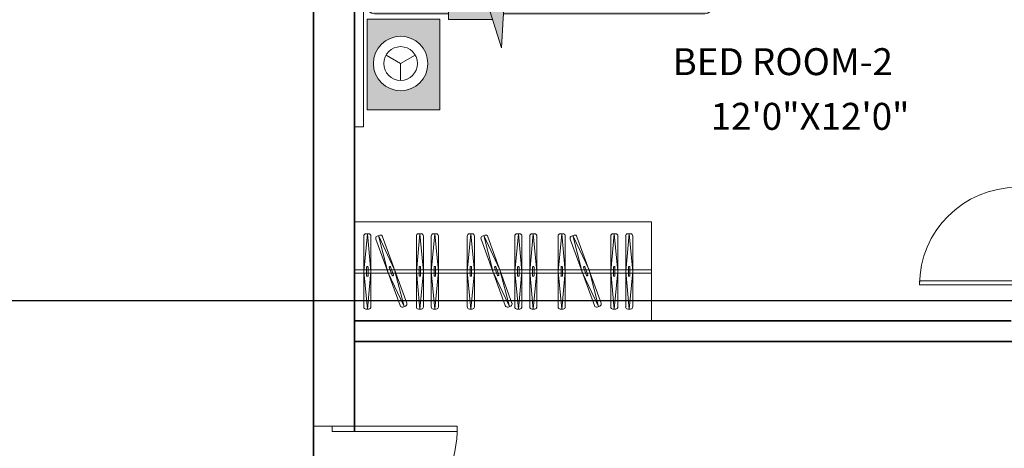
# Model space of a CAD drawing. Units: millimetres. Extents: x 27017497 to 27018854, y 7058029 to 7059154.
# Tile 79 of 91: x 27018246 to 27018462, y 7058409 to 7058503. Entities that reach past the tile are written whole.
import ezdxf

# ---------------------------------------------------------------- set-up
doc = ezdxf.new("R2010")
doc.units = ezdxf.units.MM
for name, color, linetype, lineweight in [('A-ANNO-DIMS', 2, 'Continuous', 18), ('A-AREA-IDEN', 7, 'Continuous', 18), ('A-DOOR', 4, 'Continuous', 20), ('A-FLOR-CASE', 8, 'Continuous', 20), ('A-FURN', 8, 'Continuous', 18), ('A-WALL', 7, 'Continuous', 35)]:
    doc.layers.add(name, color=color, linetype=linetype, lineweight=lineweight)
doc.layers.add('A-FURN-PATT', color=177, linetype='Continuous', lineweight=13, true_color=0x293189)
doc.styles.get("Standard").update_dxf_attribs({"font": 'arial.ttf'})
doc.dimstyles.get("Standard").update_dxf_attribs({"dimtxt": 0.18, "dimasz": 0.18, "dimexe": 0.18, "dimexo": 0.0625, "dimgap": 0.09, "dimtad": 0, "dimtih": 1, "dimtoh": 1, "dimdec": 4, "dimzin": 0, "dimdsep": 46, "dimtxsty": 'Standard', "dimcen": 0.09, "dimadec": 0, "dimazin": 0, "dimtfac": 1, "dimtdec": 4, "dimtofl": 0, "dimtmove": 0, "dimatfit": 3, "dimfxl": 1, "dimtolj": 1, "dimtzin": 0, "dimarcsym": 0})

# ---------------------------------------------------------------- blocks, each defined once
blk = doc.blocks.new('CAMMAT')
for p, q in [((1.2731, 0), (-1.2731, 0)), ((1.2731, 0), (1.2731, -0.05)), ((-1.2731, 0), (-1.2731, -0.05)), ((1.2731, -0.05), (-1.2731, -0.05)), ((-1.18, -0.07), (-1.18, -0.47)), ((-1.18, -0.07), (-0.68, -0.07)), ((-0.68, -0.07), (-0.68, -0.47)), ((0.61, -0.07), (-0.61, -0.07)), ((0.68, -0.07), (0.68, -0.47)), ((0.68, -0.07), (1.18, -0.07)), ((1.18, -0.07), (1.18, -0.47)), ((-0.65, -0.11), (-0.65, -0.5169)), ((-0.0465, -0.1395), (-0.5852, -0.1395)), ((0.5962, -0.1395), (0.0574, -0.1395)), ((0.65, -0.11), (0.65, -0.5169)), ((-0.931, -0.2541), (-0.9775, -0.1737)), ((-0.6152, -0.1695), (-0.6152, -0.4095)), ((-0.0165, -0.1695), (-0.0165, -0.4095)), ((0.0274, -0.1695), (0.0274, -0.4095)), ((0.6262, -0.1695), (0.6262, -0.4095)), ((0.9242, -0.2541), (0.8777, -0.1737)), ((-0.931, -0.2541), (-0.9775, -0.3346)), ((-0.931, -0.2541), (-0.8381, -0.2541)), ((0.9242, -0.2541), (0.8777, -0.3346)), ((0.9242, -0.2541), (1.0171, -0.2541)), ((-1.18, -0.47), (-0.68, -0.47)), ((-0.0465, -0.4395), (-0.5852, -0.4395)), ((0.5962, -0.4395), (0.0574, -0.4395)), ((0.68, -0.47), (1.18, -0.47)), ((-0.6904, -0.5169), (-0.6904, -0.8)), ((-0.6904, -0.5169), (0.6826, -0.5169)), ((0.6826, -0.5169), (0.6826, -0.7603)), ((0.0535, -0.5623), (-0.7312, -0.8093)), ((0.0535, -0.5623), (0.8382, -0.8093)), ((-0.65, -0.8139), (-0.65, -1.93)), ((0.65, -0.8204), (0.65, -1.93)), ((0.61, -1.97), (-0.61, -1.97))]:
    blk.add_line(p, q)
for points in [[(-0.1761, -1.0476), (-0.161, -0.9772), (-0.1474, -0.921), (-0.1326, -0.8732), (-0.1139, -0.8282), (-0.0886, -0.7803), (-0.0541, -0.7238), (-0.0076, -0.653), (0.0535, -0.5623)], [(0.2832, -1.0476), (0.2681, -0.9772), (0.2545, -0.921), (0.2396, -0.8732), (0.2209, -0.8282), (0.1957, -0.7803), (0.1611, -0.7238), (0.1147, -0.653), (0.0535, -0.5623)], [(-0.7312, -0.8093), (-0.5683, -0.8185), (-0.4451, -0.828), (-0.3552, -0.8406), (-0.2919, -0.8591), (-0.2489, -0.8862), (-0.2196, -0.9248), (-0.1975, -0.9777), (-0.1761, -1.0476)], [(0.8382, -0.8093), (0.6753, -0.8185), (0.5522, -0.828), (0.4622, -0.8406), (0.399, -0.8591), (0.356, -0.8862), (0.3267, -0.9248), (0.3046, -0.9777), (0.2832, -1.0476)]]:
    blk.add_lwpolyline(points)
for centre, radius in [((-0.931, -0.2541), 0.15), ((0.9242, -0.2541), 0.15), ((-0.931, -0.2541), 0.0929), ((0.9242, -0.2541), 0.0929)]:
    blk.add_circle(centre, radius)
for centre, radius, start, end in [((-0.61, -0.11), 0.04, 90, 180), ((0.61, -0.11), 0.04, 0, 90), ((-0.5852, -0.1695), 0.03, 90, 180), ((-0.0465, -0.1695), 0.03, 360, 90), ((0.0574, -0.1695), 0.03, 90, 180), ((0.5962, -0.1695), 0.03, 360, 90), ((-0.5852, -0.4095), 0.03, 180, 270), ((-0.0465, -0.4095), 0.03, 270, 360), ((0.0574, -0.4095), 0.03, 180, 270), ((0.5962, -0.4095), 0.03, 270, 360), ((-0.61, -1.93), 0.04, 180, 270), ((0.61, -1.93), 0.04, 270, 360)]:
    blk.add_arc(centre, radius, start, end)
blk = doc.blocks.new('*U2')
for p, q in [((0, 0), (0, -6)), ((40, 0), (40, -6))]:
    blk.add_line(p, q)
blk.add_lwpolyline([(0, 0), (0, 40), (1.75, 40), (1.75, 0)], close=True)
blk.add_arc((0, 0), 40, 0, 90)
blk = doc.blocks.new('WARDROBE-HANGING')
for p, q in [((0, 21.74), (65.21, 21.74)), ((0, 0), (0, 21.74)), ((65.21, 0), (65.21, 21.74)), ((4.86, 19.15), (4.08, 10.88)), ((4.08, 18.62), (4.08, 3.13)), ((5.18, 19.15), (4.55, 19.15)), ((4.86, 19.15), (5.64, 10.88)), ((5.64, 18.62), (5.64, 3.13)), ((8.14, 19.15), (7.35, 10.88)), ((7.35, 18.62), (7.35, 3.13)), ((8.45, 19.15), (7.82, 19.15)), ((8.14, 19.15), (8.92, 10.88)), ((8.92, 18.62), (8.92, 3.13)), ((16.33, 18.5), (11.03, 3.94)), ((17.8, 17.96), (12.5, 3.4)), ((17.25, 18.73), (13.68, 11.22)), ((17.25, 18.73), (15.15, 10.68)), ((17.54, 18.62), (16.95, 18.83)), ((19.66, 19.15), (18.88, 10.88)), ((18.88, 18.62), (18.88, 3.13)), ((19.98, 19.15), (19.35, 19.15)), ((19.66, 19.15), (20.45, 10.88)), ((20.45, 18.62), (20.45, 3.13)), ((25.9, 19.15), (25.12, 10.88)), ((25.12, 18.62), (25.12, 3.13)), ((26.21, 19.15), (25.59, 19.15)), ((25.9, 19.15), (26.68, 10.88)), ((26.68, 18.62), (26.68, 3.13)), ((29.17, 19.15), (28.39, 10.88)), ((28.39, 18.62), (28.39, 3.13)), ((29.49, 19.15), (28.86, 19.15)), ((29.17, 19.15), (29.96, 10.88)), ((29.96, 18.62), (29.96, 3.13)), ((35.87, 18.5), (30.57, 3.94)), ((37.34, 17.96), (32.04, 3.4)), ((36.78, 18.73), (33.22, 11.22)), ((36.78, 18.73), (34.69, 10.68)), ((37.08, 18.62), (36.49, 18.83)), ((39.59, 19.15), (38.81, 10.88)), ((38.81, 18.62), (38.81, 3.13)), ((39.9, 19.15), (39.28, 19.15)), ((39.59, 19.15), (40.37, 10.88)), ((40.37, 18.62), (40.37, 3.13)), ((47.49, 19.15), (46.71, 10.88)), ((46.71, 18.62), (46.71, 3.13)), ((47.81, 19.15), (47.18, 19.15)), ((47.49, 19.15), (48.28, 10.88)), ((48.28, 18.62), (48.28, 3.13)), ((50.77, 19.15), (49.98, 10.88)), ((49.98, 18.62), (49.98, 3.13)), ((51.08, 19.15), (50.45, 19.15)), ((50.77, 19.15), (51.55, 10.88)), ((51.55, 18.62), (51.55, 3.13)), ((58.96, 18.5), (53.66, 3.94)), ((60.43, 17.96), (55.13, 3.4)), ((59.88, 18.73), (56.31, 11.22)), ((59.88, 18.73), (57.78, 10.68)), ((60.17, 18.62), (59.58, 18.83)), ((62.29, 19.15), (61.51, 10.88)), ((61.51, 18.62), (61.51, 3.13)), ((62.61, 19.15), (61.98, 19.15)), ((62.29, 19.15), (63.08, 10.88)), ((63.08, 18.62), (63.08, 3.13)), ((0, 11.23), (65.21, 11.23)), ((4.86, 2.6), (4.08, 10.88)), ((4.71, 11.83), (4.71, 9.93)), ((4.92, 11.93), (4.8, 11.93)), ((4.86, 2.6), (5.64, 10.88)), ((5.02, 11.83), (5.02, 9.93)), ((8.14, 2.6), (7.35, 10.88)), ((7.98, 11.83), (7.98, 9.93)), ((8.2, 11.93), (8.07, 11.93)), ((8.14, 2.6), (8.92, 10.88)), ((8.29, 11.83), (8.29, 9.93)), ((11.59, 3.17), (13.68, 11.22)), ((14.59, 11.9), (13.94, 10.11)), ((14.89, 11.79), (14.24, 10)), ((14.84, 11.92), (14.72, 11.96)), ((19.66, 2.6), (18.88, 10.88)), ((19.51, 11.83), (19.51, 9.93)), ((19.73, 11.93), (19.6, 11.93)), ((19.66, 2.6), (20.45, 10.88)), ((19.82, 11.83), (19.82, 9.93)), ((25.9, 2.6), (25.12, 10.88)), ((25.74, 11.83), (25.74, 9.93)), ((25.96, 11.93), (25.84, 11.93)), ((25.9, 2.6), (26.68, 10.88)), ((26.06, 11.83), (26.06, 9.93)), ((29.17, 2.6), (28.39, 10.88)), ((29.02, 11.83), (29.02, 9.93)), ((29.24, 11.93), (29.11, 11.93)), ((29.17, 2.6), (29.96, 10.88)), ((29.33, 11.83), (29.33, 9.93)), ((31.12, 3.17), (33.22, 11.22)), ((34.13, 11.9), (33.48, 10.11)), ((34.42, 11.79), (33.77, 10)), ((34.37, 11.92), (34.25, 11.96)), ((39.59, 2.6), (38.81, 10.88)), ((39.43, 11.83), (39.43, 9.93)), ((39.65, 11.93), (39.53, 11.93)), ((39.59, 2.6), (40.37, 10.88)), ((39.75, 11.83), (39.75, 9.93)), ((47.49, 2.6), (46.71, 10.88)), ((47.34, 11.83), (47.34, 9.93)), ((47.56, 11.93), (47.43, 11.93)), ((47.49, 2.6), (48.28, 10.88)), ((47.65, 11.83), (47.65, 9.93)), ((50.77, 2.6), (49.98, 10.88)), ((50.61, 11.83), (50.61, 9.93)), ((50.83, 11.93), (50.7, 11.93)), ((50.77, 2.6), (51.55, 10.88)), ((50.92, 11.83), (50.92, 9.93)), ((54.22, 3.17), (56.31, 11.22)), ((57.22, 11.9), (56.57, 10.11)), ((57.52, 11.79), (56.87, 10)), ((57.47, 11.92), (57.35, 11.96)), ((62.29, 2.6), (61.51, 10.88)), ((62.14, 11.83), (62.14, 9.93)), ((62.36, 11.93), (62.23, 11.93)), ((62.29, 2.6), (63.08, 10.88)), ((62.45, 11.83), (62.45, 9.93)), ((0, 10.51), (65.21, 10.51)), ((4.92, 9.82), (4.8, 9.82)), ((8.2, 9.82), (8.07, 9.82)), ((11.59, 3.17), (15.15, 10.68)), ((14.11, 9.94), (14, 9.98)), ((19.73, 9.82), (19.6, 9.82)), ((25.96, 9.82), (25.84, 9.82)), ((29.24, 9.82), (29.11, 9.82)), ((31.12, 3.17), (34.69, 10.68)), ((33.65, 9.94), (33.53, 9.98)), ((39.65, 9.82), (39.53, 9.82)), ((47.56, 9.82), (47.43, 9.82)), ((50.83, 9.82), (50.7, 9.82)), ((54.22, 3.17), (57.78, 10.68)), ((56.74, 9.94), (56.63, 9.98)), ((62.36, 9.82), (62.23, 9.82)), ((5.18, 2.6), (4.55, 2.6)), ((8.45, 2.6), (7.82, 2.6)), ((11.88, 3.07), (11.29, 3.28)), ((19.98, 2.6), (19.35, 2.6)), ((26.21, 2.6), (25.59, 2.6)), ((29.49, 2.6), (28.86, 2.6)), ((31.42, 3.07), (30.83, 3.28)), ((39.9, 2.6), (39.28, 2.6)), ((47.81, 2.6), (47.18, 2.6)), ((51.08, 2.6), (50.45, 2.6)), ((54.51, 3.07), (53.92, 3.28)), ((62.61, 2.6), (61.98, 2.6)), ((0, 0), (65.21, 0))]:
    blk.add_line(p, q)
for centre, major_axis, start_param, end_param in [((4.55, 18.62), (0, 0.528), 0, 1.570796), ((5.18, 18.62), (0, 0.528), 4.712389, 6.283185), ((7.82, 18.62), (0, 0.528), 0, 1.570796), ((8.45, 18.62), (0, 0.528), 4.712389, 6.283185), ((16.77, 18.34), (0.181, 0.496), 0, 1.570796), ((17.36, 18.12), (0.181, 0.496), -1.570796, 0), ((19.35, 18.62), (0, 0.528), 0, 1.570796), ((19.98, 18.62), (0, 0.528), 4.712389, 6.283185), ((25.59, 18.62), (0, 0.528), 0, 1.570796), ((26.21, 18.62), (0, 0.528), 4.712389, 6.283185), ((28.86, 18.62), (0, 0.528), 0, 1.570796), ((29.49, 18.62), (0, 0.528), 4.712389, 6.283185), ((36.31, 18.34), (0.181, 0.496), 0, 1.570796), ((36.9, 18.12), (0.181, 0.496), -1.570796, 0), ((39.28, 18.62), (0, 0.528), 0, 1.570796), ((39.9, 18.62), (0, 0.528), 4.712389, 6.283185), ((47.18, 18.62), (0, 0.528), 0, 1.570796), ((47.81, 18.62), (0, 0.528), 4.712389, 6.283185), ((50.45, 18.62), (0, 0.528), 0, 1.570796), ((51.08, 18.62), (0, 0.528), 4.712389, 6.283185), ((59.4, 18.34), (0.181, 0.496), 0, 1.570796), ((59.99, 18.12), (0.181, 0.496), -1.570796, 0), ((61.98, 18.62), (0, 0.528), 0, 1.570796), ((62.61, 18.62), (0, 0.528), 4.712389, 6.283185), ((4.8, 11.83), (0, 0.106), 0, 1.570796), ((4.92, 11.83), (0, 0.106), -1.570796, 0), ((8.07, 11.83), (0, 0.106), 0, 1.570796), ((8.2, 11.83), (0, 0.106), -1.570796, 0), ((14.68, 11.86), (0.0361, 0.0993), 0, 1.570796), ((14.8, 11.82), (0.0361, 0.0993), 4.712389, 6.283185), ((19.6, 11.83), (0, 0.106), 0, 1.570796), ((19.73, 11.83), (0, 0.106), -1.570796, 0), ((25.84, 11.83), (0, 0.106), 0, 1.570796), ((25.96, 11.83), (0, 0.106), -1.570796, 0), ((29.11, 11.83), (0, 0.106), 0, 1.570796), ((29.24, 11.83), (0, 0.106), -1.570796, 0), ((34.22, 11.86), (0.0361, 0.0993), 0, 1.570796), ((34.34, 11.82), (0.0361, 0.0993), 4.712389, 6.283185), ((39.53, 11.83), (0, 0.106), 0, 1.570796), ((39.65, 11.83), (0, 0.106), -1.570796, 0), ((47.43, 11.83), (0, 0.106), 0, 1.570796), ((47.56, 11.83), (0, 0.106), -1.570796, 0), ((50.7, 11.83), (0, 0.106), 0, 1.570796), ((50.83, 11.83), (0, 0.106), -1.570796, 0), ((57.31, 11.86), (0.0361, 0.0993), 0, 1.570796), ((57.43, 11.82), (0.0361, 0.0993), 4.712389, 6.283185), ((62.23, 11.83), (0, 0.106), 0, 1.570796), ((62.36, 11.83), (0, 0.106), -1.570796, 0), ((4.8, 9.93), (0, 0.106), 1.570796, 3.141593), ((4.92, 9.93), (0, 0.106), 3.141593, 4.712389), ((8.07, 9.93), (0, 0.106), 1.570796, 3.141593), ((8.2, 9.93), (0, 0.106), 3.141593, 4.712389), ((14.03, 10.08), (0.0361, 0.0993), 1.570796, 3.141593), ((14.15, 10.03), (0.0361, 0.0993), 3.141593, 4.712389), ((19.6, 9.93), (0, 0.106), 1.570796, 3.141593), ((19.73, 9.93), (0, 0.106), 3.141593, 4.712389), ((25.84, 9.93), (0, 0.106), 1.570796, 3.141593), ((25.96, 9.93), (0, 0.106), 3.141593, 4.712389), ((29.11, 9.93), (0, 0.106), 1.570796, 3.141593), ((29.24, 9.93), (0, 0.106), 3.141593, 4.712389), ((33.57, 10.08), (0.0361, 0.0993), 1.570796, 3.141593), ((33.69, 10.03), (0.0361, 0.0993), 3.141593, 4.712389), ((39.53, 9.93), (0, 0.106), 1.570796, 3.141593), ((39.65, 9.93), (0, 0.106), 3.141593, 4.712389), ((47.43, 9.93), (0, 0.106), 1.570796, 3.141593), ((47.56, 9.93), (0, 0.106), 3.141593, 4.712389), ((50.7, 9.93), (0, 0.106), 1.570796, 3.141593), ((50.83, 9.93), (0, 0.106), 3.141593, 4.712389), ((56.66, 10.08), (0.0361, 0.0993), 1.570796, 3.141593), ((56.78, 10.03), (0.0361, 0.0993), 3.141593, 4.712389), ((62.23, 9.93), (0, 0.106), 1.570796, 3.141593), ((62.36, 9.93), (0, 0.106), 3.141593, 4.712389), ((4.55, 3.13), (0, 0.528), 1.570796, 3.141593), ((5.18, 3.13), (0, 0.528), 3.141593, 4.712389), ((7.82, 3.13), (0, 0.528), 1.570796, 3.141593), ((8.45, 3.13), (0, 0.528), 3.141593, 4.712389), ((11.47, 3.78), (0.181, 0.496), 1.570796, 3.141593), ((12.06, 3.56), (0.181, 0.496), 3.141593, 4.712389), ((19.35, 3.13), (0, 0.528), 1.570796, 3.141593), ((19.98, 3.13), (0, 0.528), 3.141593, 4.712389), ((25.59, 3.13), (0, 0.528), 1.570796, 3.141593), ((26.21, 3.13), (0, 0.528), 3.141593, 4.712389), ((28.86, 3.13), (0, 0.528), 1.570796, 3.141593), ((29.49, 3.13), (0, 0.528), 3.141593, 4.712389), ((31.01, 3.78), (0.181, 0.496), 1.570796, 3.141593), ((31.6, 3.56), (0.181, 0.496), 3.141593, 4.712389), ((39.28, 3.13), (0, 0.528), 1.570796, 3.141593), ((39.9, 3.13), (0, 0.528), 3.141593, 4.712389), ((47.18, 3.13), (0, 0.528), 1.570796, 3.141593), ((47.81, 3.13), (0, 0.528), 3.141593, 4.712389), ((50.45, 3.13), (0, 0.528), 1.570796, 3.141593), ((51.08, 3.13), (0, 0.528), 3.141593, 4.712389), ((54.1, 3.78), (0.181, 0.496), 1.570796, 3.141593), ((54.69, 3.56), (0.181, 0.496), 3.141593, 4.712389), ((61.98, 3.13), (0, 0.528), 1.570796, 3.141593), ((62.61, 3.13), (0, 0.528), 3.141593, 4.712389)]:
    blk.add_ellipse(centre, major_axis=major_axis, ratio=0.888892, start_param=start_param, end_param=end_param)
blk = doc.blocks.new('*D48')
at = {"layer": 'A-ANNO-DIMS', "color": 0, "lineweight": -2, "transparency": 16777216}
for p, q in [((27018463.5, 7058622.91), (27017497.54, 7058622.91)), ((27017497.72, 7058622.73), (27017497.72, 7058357.75)), ((27017497.72, 7058092.41), (27017497.72, 7058357.39)), ((27018555.13, 7058092.23), (27017497.54, 7058092.23))]:
    blk.add_line(p, q, dxfattribs=at)
at = {"layer": 'A-ANNO-DIMS', "color": 0, "transparency": 16777216}
for points in [[(27017497.69, 7058622.73), (27017497.75, 7058622.73), (27017497.72, 7058622.91)], [(27017497.69, 7058092.41), (27017497.75, 7058092.41), (27017497.72, 7058092.23)]]:
    blk.add_solid(points, dxfattribs=at)
at = {"layer": 'Defpoints', "color": 0, "transparency": 16777216}
for p in [(27018463.56, 7058622.91), (27017497.72, 7058092.23), (27018555.19, 7058092.23)]:
    blk.add_point(p, dxfattribs=at)
at = {"layer": 'A-ANNO-DIMS', "color": 0, "transparency": 16777216, "insert": (27017497.72, 7058357.57), "char_height": 0.18, "attachment_point": 5}
blk.add_mtext('\\A1;530.7', dxfattribs=at)
blk = doc.blocks.new('*D50')
at = {"layer": 'A-ANNO-DIMS', "color": 0, "lineweight": -2, "transparency": 16777216}
for p, q in [((27018223.67, 7058580.91), (27018854.24, 7058580.91)), ((27018854.06, 7058580.73), (27018854.06, 7058511.34)), ((27018854.06, 7058441.59), (27018854.06, 7058510.98)), ((27018223.67, 7058441.41), (27018854.24, 7058441.41))]:
    blk.add_line(p, q, dxfattribs=at)
at = {"layer": 'A-ANNO-DIMS', "color": 0, "transparency": 16777216}
for points in [[(27018854.03, 7058580.73), (27018854.09, 7058580.73), (27018854.06, 7058580.91)], [(27018854.03, 7058441.59), (27018854.09, 7058441.59), (27018854.06, 7058441.41)]]:
    blk.add_solid(points, dxfattribs=at)
at = {"layer": 'Defpoints', "color": 0, "transparency": 16777216}
for p in [(27018223.61, 7058580.91), (27018223.61, 7058441.41), (27018854.06, 7058441.41)]:
    blk.add_point(p, dxfattribs=at)
at = {"layer": 'A-ANNO-DIMS', "color": 0, "transparency": 16777216, "insert": (27018854.06, 7058511.16), "char_height": 0.18, "attachment_point": 5}
blk.add_mtext('\\A1;139.5', dxfattribs=at)

msp = doc.modelspace()

# ---------------------------------------------------------------- hatches: boundary and pattern name
at = {"layer": 'A-FURN-PATT'}
h = msp.add_hatch(color=256, dxfattribs=at)
h.dxf.hatch_style = 1
h.paths.add_polyline_path([(27018398.067, 7058554.497, 0.4142136), (27018396.474, 7058556.09), (27018352.018, 7058556.09), (27018352.202, 7058552.834), (27018352.581, 7058547.929), (27018353.082, 7058544.346), (27018353.818, 7058541.828), (27018354.899, 7058540.115), (27018356.437, 7058538.948), (27018358.543, 7058538.068), (27018361.329, 7058537.215), (27018358.524, 7058536.613), (27018356.284, 7058536.07), (27018354.381, 7058535.48), (27018352.588, 7058534.736), (27018350.68, 7058533.729), (27018348.431, 7058532.354), (27018345.612, 7058530.503), (27018341.998, 7058528.068), (27018345.612, 7058525.633), (27018348.431, 7058523.782), (27018350.68, 7058522.407), (27018352.588, 7058521.4), (27018354.381, 7058520.656), (27018356.284, 7058520.066), (27018358.524, 7058519.523), (27018361.329, 7058518.92), (27018358.543, 7058518.068), (27018356.437, 7058517.188), (27018354.899, 7058516.021), (27018353.818, 7058514.308), (27018353.082, 7058511.79), (27018352.581, 7058508.207), (27018352.28, 7058504.311), (27018396.474, 7058504.311, 0.4142136), (27018398.067, 7058505.904)])
h.paths.add_polyline_path([(27018356.437, 7058538.948), (27018354.899, 7058540.115), (27018353.818, 7058541.828), (27018353.082, 7058544.346), (27018352.581, 7058547.929), (27018352.202, 7058552.834), (27018351.835, 7058559.322), (27018341.998, 7058528.068), (27018345.612, 7058530.503), (27018348.431, 7058532.354), (27018350.68, 7058533.729), (27018352.588, 7058534.736), (27018354.381, 7058535.48), (27018356.284, 7058536.07), (27018358.524, 7058536.613), (27018361.329, 7058537.215), (27018358.543, 7058538.068)])
h.paths.add_polyline_path([(27018358.543, 7058518.068), (27018361.329, 7058518.92), (27018358.524, 7058519.523), (27018356.284, 7058520.066), (27018354.381, 7058520.656), (27018352.588, 7058521.4), (27018350.68, 7058522.407), (27018348.431, 7058523.782), (27018345.612, 7058525.633), (27018341.998, 7058528.068), (27018351.835, 7058496.813), (27018352.202, 7058503.301), (27018352.581, 7058508.207), (27018353.082, 7058511.79), (27018353.818, 7058514.308), (27018354.899, 7058516.021), (27018356.437, 7058517.188)])
h.paths.add_polyline_path([(27018351.324, 7058557.699), (27018340.191, 7058557.699), (27018340.191, 7058503.014), (27018349.884, 7058503.014), (27018341.998, 7058528.068)])
h.paths.add_polyline_path([(27018340.191, 7058556.09), (27018323.983, 7058556.09, 0.4142136), (27018322.39, 7058554.497), (27018322.39, 7058505.904, 0.4142136), (27018323.983, 7058504.311), (27018340.191, 7058504.311)])
h.paths.add_polyline_path([(27018337.107, 7058532.051, -0.4142136), (27018335.912, 7058530.856), (27018326.353, 7058530.856, -0.4142136), (27018325.158, 7058532.051), (27018325.158, 7058553.51, -0.4142136), (27018326.353, 7058554.705), (27018335.912, 7058554.705, -0.4142136), (27018337.107, 7058553.51)], flags=0)
h.paths.add_polyline_path([(27018337.107, 7058527.914), (27018337.107, 7058506.454, -0.4142136), (27018335.912, 7058505.259), (27018326.353, 7058505.259, -0.4142136), (27018325.158, 7058506.454), (27018325.158, 7058527.914, -0.4142136), (27018326.353, 7058529.109), (27018335.912, 7058529.109, -0.4142136)], flags=0)
h.paths.add_polyline_path([(27018338.322, 7058577.2), (27018322.39, 7058577.2), (27018322.39, 7058557.285), (27018338.322, 7058557.285)])
h.paths.add_polyline_path([(27018323.748, 7058567.284, -1), (27018335.697, 7058567.284, -1)], flags=16)
h.paths.add_polyline_path([(27018326.023, 7058567.284, -1), (27018333.423, 7058567.284, -1)], flags=0)
h.paths.add_polyline_path([(27018338.322, 7058503.116), (27018322.39, 7058503.116), (27018322.39, 7058483.201), (27018338.322, 7058483.201)])
h.paths.add_polyline_path([(27018335.697, 7058493.391, -1), (27018323.748, 7058493.391, -1)], flags=16)
h.paths.add_polyline_path([(27018333.423, 7058493.391, -1), (27018326.023, 7058493.391, -1)], flags=0)
h.paths.add_polyline_path([(27018337.107, 7058527.914, 0.4142136), (27018335.912, 7058529.109), (27018326.353, 7058529.109, 0.4142136), (27018325.158, 7058527.914), (27018325.158, 7058506.454, 0.4142136), (27018326.353, 7058505.259), (27018335.912, 7058505.259, 0.4142136), (27018337.107, 7058506.454)], flags=16)
h.paths.add_polyline_path([(27018337.107, 7058553.51, 0.4142136), (27018335.912, 7058554.705), (27018326.353, 7058554.705, 0.4142136), (27018325.158, 7058553.51), (27018325.158, 7058532.051, 0.4142136), (27018326.353, 7058530.856), (27018335.912, 7058530.856, 0.4142136), (27018337.107, 7058532.051)], flags=16)

# ---------------------------------------------------------------- linework, layer by layer
at = {"layer": 'A-WALL'}
for p, q in [((27018310.606, 7058589.912), (27018310.606, 7058413.839)), ((27018310.606, 7058589.912), (27018310.606, 7058169.223)), ((27018319.606, 7058580.912), (27018319.606, 7058412.636)), ((27018463.606, 7058436.912), (27018319.606, 7058436.912)), ((27018468.106, 7058432.412), (27018319.606, 7058432.412))]:
    msp.add_line(p, q, dxfattribs=at)

# ---------------------------------------------------------------- block references
at = {"layer": 'A-DOOR'}
for p, xscale, yscale, zscale, rotation in [((27018464.924, 7058444.814), 0.5347783892510444, 0.5347783892510444, 0.5347783892510444, 90.00000000000003), ((27018314.676, 7058413.839), 0.6870473523349573, 0.6870473523349573, 0.6870473523349573, 270)]:
    msp.add_blockref('*U2', p, dxfattribs=dict(at, xscale=xscale, yscale=yscale, zscale=zscale, rotation=rotation))
at = {"layer": 'A-FLOR-CASE', "extrusion": (0, 0, -1), "zscale": -1}
msp.add_blockref('WARDROBE-HANGING', (-27018384.717, 7058436.905), dxfattribs=at)
at = {"layer": 'A-FURN', "xscale": -39.82996475819422, "yscale": 39.82996475819422, "zscale": 39.82996475819422, "rotation": 90}
msp.add_blockref('CAMMAT', (27018319.602, 7058530.2), dxfattribs=at)

# ---------------------------------------------------------------- texts
at = {"layer": 'A-ANNO-DIMS'}
msp.add_text('12\'0"X12\'0"', height=5.91176, dxfattribs=at).set_placement((27018397.723, 7058478.846))
at = {"layer": 'A-AREA-IDEN'}
msp.add_text('BED ROOM-2', height=5.9118, dxfattribs=at).set_placement((27018389.375, 7058490.843))

# ---------------------------------------------------------------- dimensions: what is measured, and where the dimension line sits
at = {"layer": 'A-ANNO-DIMS'}
for base, p1, p2, picture, middle in [((27017497.716, 7058092.23), (27018463.561, 7058622.912), (27018555.192, 7058092.23), '*D48', (27017497.716, 7058357.571)), ((27018854.056, 7058441.412), (27018223.606, 7058580.912), (27018223.606, 7058441.412), '*D50', (27018854.056, 7058511.162))]:
    dim = msp.add_linear_dim(base=base, p1=p1, p2=p2, angle=90, dimstyle='Standard', override={"dimdec": 1, "dimlfac": 1, "dimrnd": 0, "dimzin": 0, "dimdsep": 46, "dimlunit": 2}, dxfattribs=at)
    dim.commit()
    dim.dimension.update_dxf_attribs({"geometry": picture, "text_midpoint": middle})

doc.saveas('drawing.dxf')
